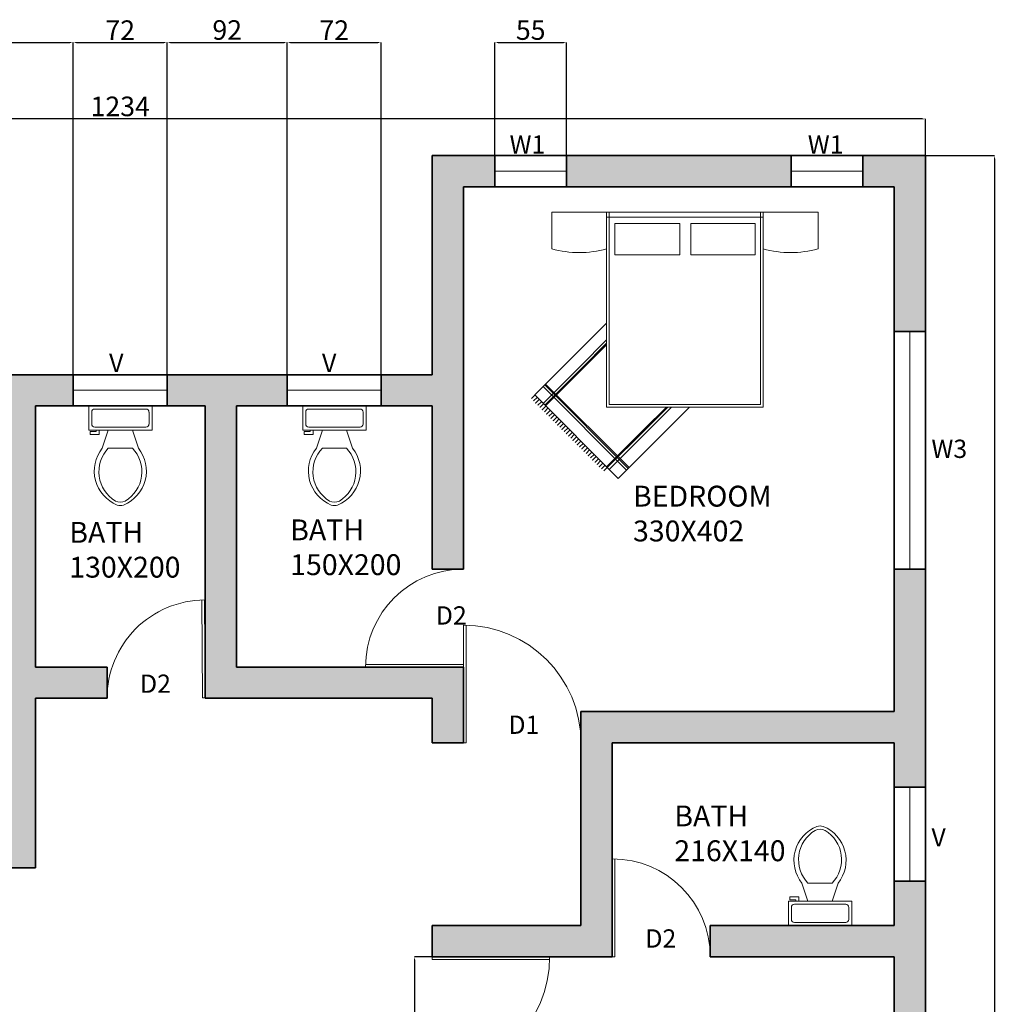
# Model space of a CAD drawing. Units: centimetres. Extents: x 2449 to 7478, y 778 to 2486.
# Tile 9 of 9: x 6695 to 7444, y 1732 to 2486. Entities that reach past the tile are written whole.
import ezdxf

# ---------------------------------------------------------------- set-up
doc = ezdxf.new("R2010")
doc.units = ezdxf.units.CM
for name, color, linetype, lineweight in [('A-ANNO-DIMS', 2, 'Continuous', 18), ('A-ANNO-TEXT', 7, 'Continuous', 18), ('A-AREA-IDEN', 7, 'Continuous', 18), ('A-DOOR', 4, 'Continuous', 18), ('A-FLOR-FIXT', 8, 'Continuous', 18), ('A-WALL', 7, 'Continuous', 35), ('A-WALL-PATT', 7, 'Continuous', 13), ('B-FURNITURE', 22, 'Continuous', 18), ('Win', 1, 'Continuous', 18)]:
    doc.layers.add(name, color=color, linetype=linetype, lineweight=lineweight)
doc.styles.get("Standard").update_dxf_attribs({"font": 'arial.ttf'})
doc.dimstyles.new('ISO-25', dxfattribs={"dimtxt": 15, "dimasz": 2.5, "dimexe": 0, "dimexo": 0, "dimgap": 0, "dimtad": 1, "dimtxsty": 'Standard', "dimcen": 2.5, "dimadec": 0, "dimazin": 0, "dimtfac": 1, "dimtmove": 0, "dimatfit": 3, "dimfxl": 1, "dimarcsym": 0})

# ---------------------------------------------------------------- blocks, each defined once
blk = doc.blocks.new('Toilet - top')
for p, q in [((9.5, -6), (9.5, -2)), ((-10, -8.5), (-8, -8.5)), ((-10, -9.5), (-10, -8.5)), ((-7, -9.5), (-10, -9.5)), ((-8, -8.5), (-8, -8)), ((-7, -8), (-7, -9.5)), ((-4, -8), (-6, -14)), ((4, -8), (6, -14)), ((4, -14), (-4, -14))]:
    blk.add_line(p, q)
blk.add_lwpolyline([(10.5, -8), (10.5, 0), (-10.5, 0), (-10.5, -8)], close=True)
for points in [[(-9.5, -2), (-9.5, -6)], [(8.5, -1), (-8.5, -1)], [(-8.5, -7), (8.5, -7)]]:
    blk.add_lwpolyline(points)
for centre, radius, start, end in [((-8.62, -1.88), 0.884, 81.8699, 188.1301), ((8.62, -1.88), 0.884, 351.8699, 98.1301), ((-8.62, -6.12), 0.884, 171.8699, 278.1301), ((8.62, -6.12), 0.884, 261.8699, 8.1301), ((3.52, -21.58), 12.17, 141.4691, 247.9714), ((4.2, -21.82), 11.33, 136.3677, 238.9468), ((-3.52, -21.58), 12.17, 292.0284, 38.5307), ((-4.2, -21.82), 11.33, 301.053, 43.6321), ((0, -27.88), 4, 245.7318, 294.2682), ((0, -29), 4, 254.8605, 285.1395)]:
    blk.add_arc(centre, radius, start, end)
blk = doc.blocks.new('A$C376C2187')
at = {"layer": 'B-FURNITURE'}
for p, q in [((-1.53, 1.82), (-1.53, 2.24)), ((-1.53, 2.24), (-0.9, 2.24)), ((-0.9, 0), (-0.9, 2.24)), ((-0.9, 2.24), (0.9, 2.24)), ((-0.9, 2.24), (-0.9, 1.82)), ((-0.9, 2.182), (0.9, 2.182)), ((-0.87, 0.03), (-0.87, 2.24)), ((0.87, 2.24), (0.87, 0.03)), ((0.9, 2.24), (0.9, 0)), ((0.9, 1.82), (0.9, 2.24)), ((0.9, 2.24), (1.53, 2.24)), ((1.53, 2.24), (1.53, 1.82)), ((-0.807, 2.112), (-0.057, 2.112)), ((-0.807, 1.749), (-0.807, 2.112)), ((-0.057, 2.112), (-0.057, 1.749)), ((0.069, 2.112), (0.807, 2.112)), ((0.069, 2.112), (0.069, 1.749)), ((0.807, 2.112), (0.807, 1.749)), ((-0.807, 1.749), (-0.057, 1.749)), ((0.069, 1.749), (0.807, 1.749)), ((0.9, 0), (-0.9, 0)), ((0.87, 0.03), (-0.87, 0.03))]:
    blk.add_line(p, q, dxfattribs=at)
for centre in [(-1.215, 2.926), (1.215, 2.926)]:
    blk.add_arc(centre, 1.15, 254.0965, 285.9035, dxfattribs=at)
blk = doc.blocks.new('3')
for p, q in [((5936.31, 1821.57), (5936.31, 1746.57)), ((5938.31, 1821.57), (5938.31, 1746.57)), ((5938.31, 1746.57), (5936.31, 1746.57))]:
    blk.add_line(p, q)
blk.add_arc((5936.31, 1746.57), 75, 0, 90)
blk = doc.blocks.new('2')
for p, q in [((5717.35, 1812.71), (5717.35, 1722.71)), ((5719.35, 1812.71), (5719.35, 1722.71)), ((5719.35, 1722.71), (5717.35, 1722.71))]:
    blk.add_line(p, q)
blk.add_arc((5717.35, 1722.71), 90, 0, 90)
blk = doc.blocks.new('*D63')
at = {"layer": 'A-ANNO-DIMS', "color": 0, "lineweight": -2, "transparency": 16777216}
for p, q in [((6155.01, 2214.34), (6155.01, 2410.3)), ((7386.51, 2410.3), (6157.51, 2410.3)), ((7389.01, 2382.34), (7389.01, 2410.3))]:
    blk.add_line(p, q, dxfattribs=at)
at = {"layer": 'A-ANNO-DIMS', "color": 0, "transparency": 16777216}
for points in [[(6157.51, 2410.71), (6157.51, 2409.88), (6155.01, 2410.3)], [(7386.51, 2410.71), (7386.51, 2409.88), (7389.01, 2410.3)]]:
    blk.add_solid(points, dxfattribs=at)
at = {"layer": 'Defpoints', "color": 0, "transparency": 16777216}
for p in [(6155.01, 2410.3), (7389.01, 2382.34), (6155.01, 2214.34)]:
    blk.add_point(p, dxfattribs=at)
at = {"layer": 'A-ANNO-DIMS', "color": 0, "transparency": 16777216, "insert": (6772.01, 2417.96), "char_height": 15, "attachment_point": 5}
blk.add_mtext('1234', dxfattribs=at)
blk = doc.blocks.new('*D64')
at = {"layer": 'A-ANNO-DIMS', "color": 0, "lineweight": -2, "transparency": 16777216}
for p, q in [((7389.01, 2382.34), (7441.8, 2382.34)), ((7441.8, 2379.84), (7441.8, 1022.84)), ((7389.01, 1020.34), (7441.8, 1020.34))]:
    blk.add_line(p, q, dxfattribs=at)
at = {"layer": 'A-ANNO-DIMS', "color": 0, "transparency": 16777216}
for points in [[(7441.38, 2379.84), (7442.21, 2379.84), (7441.8, 2382.34)], [(7441.38, 1022.84), (7442.21, 1022.84), (7441.8, 1020.34)]]:
    blk.add_solid(points, dxfattribs=at)
at = {"layer": 'Defpoints', "color": 0, "transparency": 16777216}
for p in [(7389.01, 2382.34), (7389.01, 1020.34), (7441.8, 1020.34)]:
    blk.add_point(p, dxfattribs=at)
at = {"layer": 'A-ANNO-DIMS', "color": 0, "transparency": 16777216, "insert": (7434.13, 1701.34), "char_height": 15, "attachment_point": 5, "rotation": 90}
blk.add_mtext('1362', dxfattribs=at)
blk = doc.blocks.new('RUG-FRINGED-A')
for p, q in [((57.64, 119.07), (31.14, 92.56)), ((37.52, 86.17), (57.64, 106.29)), ((38.88, 84.82), (57.64, 103.58)), ((39.46, 84.24), (57.64, 102.42)), ((2.52, 63.95), (31.14, 92.56)), ((37.52, 86.17), (8.91, 57.56)), ((38.88, 84.82), (10.26, 56.2)), ((39.46, 84.24), (10.84, 55.62)), ((72.85, 6.39), (8.91, 70.34)), ((74.21, 7.74), (10.26, 71.69)), ((74.79, 8.33), (10.84, 72.27)), ((2.62, 63.84), (0, 61.22)), ((4.3, 62.16), (1.68, 59.54)), ((66.47, 0), (2.52, 63.95)), ((5.98, 60.48), (3.36, 57.86)), ((7.66, 58.8), (5.04, 56.18)), ((9.34, 57.12), (6.72, 54.5)), ((11.02, 55.44), (8.4, 52.82)), ((12.7, 53.76), (10.08, 51.14)), ((103.41, 54.71), (86.2, 37.5)), ((104.58, 54.71), (86.78, 36.92)), ((107.29, 54.71), (88.14, 35.56)), ((95.08, 28.62), (121.18, 54.71)), ((14.38, 52.08), (11.76, 49.46)), ((16.06, 50.4), (13.44, 47.78)), ((17.74, 48.72), (15.12, 46.1)), ((19.42, 47.04), (16.8, 44.42)), ((21.1, 45.36), (18.48, 42.74)), ((22.78, 43.68), (20.16, 41.06)), ((24.46, 42), (21.84, 39.38)), ((26.14, 40.32), (23.52, 37.7)), ((27.82, 38.64), (25.2, 36.02)), ((29.5, 36.96), (26.88, 34.34)), ((31.18, 35.28), (28.56, 32.66)), ((32.86, 33.6), (30.24, 30.98)), ((34.54, 31.92), (31.92, 29.3)), ((36.22, 30.24), (33.6, 27.62)), ((57.58, 8.88), (86.2, 37.5)), ((58.16, 8.3), (86.78, 36.92)), ((59.52, 6.95), (88.14, 35.56)), ((37.9, 28.56), (35.28, 25.94)), ((39.58, 26.88), (36.96, 24.26)), ((41.26, 25.2), (38.64, 22.58)), ((42.94, 23.52), (40.32, 20.9)), ((95.08, 28.62), (66.47, 0)), ((44.62, 21.84), (42, 19.22)), ((46.3, 20.16), (43.68, 17.54)), ((47.98, 18.48), (45.36, 15.86)), ((49.66, 16.8), (47.04, 14.18)), ((51.34, 15.12), (48.72, 12.5)), ((53.02, 13.44), (50.4, 10.82)), ((54.7, 11.76), (52.08, 9.14)), ((56.38, 10.08), (53.76, 7.46)), ((58.07, 8.4), (55.44, 5.78))]:
    blk.add_line(p, q)
for centre in [(1.62, 59.48), (3.3, 57.8), (4.98, 56.12), (6.66, 54.44), (8.34, 52.76), (10.02, 51.08), (11.7, 49.4), (13.38, 47.72), (15.06, 46.04), (16.74, 44.36), (18.42, 42.68), (20.1, 41), (21.78, 39.32), (23.46, 37.64), (25.14, 35.96), (26.82, 34.28), (28.5, 32.6), (30.18, 30.92), (31.86, 29.24), (33.54, 27.56), (35.22, 25.88), (36.9, 24.2), (38.58, 22.52), (40.26, 20.84), (41.94, 19.16), (43.62, 17.48), (45.3, 15.8), (46.98, 14.12), (48.66, 12.44), (50.34, 10.76), (52.02, 9.08)]:
    blk.add_circle(centre, 0.0789)
blk = doc.blocks.new('*D74')
at = {"layer": 'A-ANNO-DIMS', "color": 0, "lineweight": -2, "transparency": 16777216}
for p, q in [((7011.01, 1768.34), (6997.51, 1768.34)), ((6997.51, 1765.84), (6997.51, 1680.84)), ((7011.01, 1678.34), (6997.51, 1678.34)), ((6997.51, 1678.34), (6997.51, 1502.28))]:
    blk.add_line(p, q, dxfattribs=at)
at = {"layer": 'A-ANNO-DIMS', "color": 0, "transparency": 16777216}
for points in [[(6997.09, 1765.84), (6997.92, 1765.84), (6997.51, 1768.34)], [(6997.09, 1680.84), (6997.92, 1680.84), (6997.51, 1678.34)]]:
    blk.add_solid(points, dxfattribs=at)
at = {"layer": 'Defpoints', "color": 0, "transparency": 16777216}
for p in [(7011.01, 1768.34), (6997.51, 1678.34), (7011.01, 1678.34)]:
    blk.add_point(p, dxfattribs=at)
at = {"layer": 'A-ANNO-DIMS', "color": 0, "transparency": 16777216, "insert": (6989.75, 1589.06), "char_height": 15, "attachment_point": 5, "rotation": 90}
blk.add_mtext('DOOR D1 90 TYP.', dxfattribs=at)
blk = doc.blocks.new('*D109')
at = {"layer": 'A-ANNO-DIMS', "color": 0, "lineweight": -2, "transparency": 16777216}
for p, q in [((6609.01, 2214.34), (6609.01, 2468.84)), ((6611.51, 2468.84), (6733.51, 2468.84)), ((6736.01, 2214.34), (6736.01, 2468.84))]:
    blk.add_line(p, q, dxfattribs=at)
at = {"layer": 'A-ANNO-DIMS', "color": 0, "transparency": 16777216}
for points in [[(6611.51, 2469.26), (6611.51, 2468.42), (6609.01, 2468.84)], [(6733.51, 2469.26), (6733.51, 2468.42), (6736.01, 2468.84)]]:
    blk.add_solid(points, dxfattribs=at)
at = {"layer": 'Defpoints', "color": 0, "transparency": 16777216}
for p in [(6736.01, 2468.84), (6609.01, 2214.34), (6736.01, 2214.34)]:
    blk.add_point(p, dxfattribs=at)
at = {"layer": 'A-ANNO-DIMS', "color": 0, "transparency": 16777216, "insert": (6672.51, 2476.37), "char_height": 15, "attachment_point": 5}
blk.add_mtext('127', dxfattribs=at)
blk = doc.blocks.new('*D110')
at = {"layer": 'A-ANNO-DIMS', "color": 0, "lineweight": -2, "transparency": 16777216}
for p, q in [((6736.01, 2214.34), (6736.01, 2468.84)), ((6738.51, 2468.84), (6805.51, 2468.84)), ((6808.01, 2214.34), (6808.01, 2468.84))]:
    blk.add_line(p, q, dxfattribs=at)
at = {"layer": 'A-ANNO-DIMS', "color": 0, "transparency": 16777216}
for points in [[(6738.51, 2469.26), (6738.51, 2468.42), (6736.01, 2468.84)], [(6805.51, 2469.26), (6805.51, 2468.42), (6808.01, 2468.84)]]:
    blk.add_solid(points, dxfattribs=at)
at = {"layer": 'Defpoints', "color": 0, "transparency": 16777216}
for p in [(6808.01, 2468.84), (6736.01, 2214.34), (6808.01, 2214.34)]:
    blk.add_point(p, dxfattribs=at)
at = {"layer": 'A-ANNO-DIMS', "color": 0, "transparency": 16777216, "insert": (6772.01, 2476.37), "char_height": 15, "attachment_point": 5}
blk.add_mtext('72', dxfattribs=at)
blk = doc.blocks.new('*D111')
at = {"layer": 'A-ANNO-DIMS', "color": 0, "lineweight": -2, "transparency": 16777216}
for p, q in [((6808.01, 2214.34), (6808.01, 2468.84)), ((6810.51, 2468.84), (6897.51, 2468.84)), ((6900.01, 2214.34), (6900.01, 2468.84))]:
    blk.add_line(p, q, dxfattribs=at)
at = {"layer": 'A-ANNO-DIMS', "color": 0, "transparency": 16777216}
for points in [[(6810.51, 2469.26), (6810.51, 2468.42), (6808.01, 2468.84)], [(6897.51, 2469.26), (6897.51, 2468.42), (6900.01, 2468.84)]]:
    blk.add_solid(points, dxfattribs=at)
at = {"layer": 'Defpoints', "color": 0, "transparency": 16777216}
for p in [(6900.01, 2468.84), (6808.01, 2214.34), (6900.01, 2214.34)]:
    blk.add_point(p, dxfattribs=at)
at = {"layer": 'A-ANNO-DIMS', "color": 0, "transparency": 16777216, "insert": (6854.01, 2476.5), "char_height": 15, "attachment_point": 5}
blk.add_mtext('92', dxfattribs=at)
blk = doc.blocks.new('*D112')
at = {"layer": 'A-ANNO-DIMS', "color": 0, "lineweight": -2, "transparency": 16777216}
for p, q in [((6900.01, 2214.34), (6900.01, 2468.84)), ((6902.51, 2468.84), (6969.51, 2468.84)), ((6972.01, 2214.34), (6972.01, 2468.84))]:
    blk.add_line(p, q, dxfattribs=at)
at = {"layer": 'A-ANNO-DIMS', "color": 0, "transparency": 16777216}
for points in [[(6902.51, 2469.26), (6902.51, 2468.42), (6900.01, 2468.84)], [(6969.51, 2469.26), (6969.51, 2468.42), (6972.01, 2468.84)]]:
    blk.add_solid(points, dxfattribs=at)
at = {"layer": 'Defpoints', "color": 0, "transparency": 16777216}
for p in [(6972.01, 2468.84), (6900.01, 2214.34), (6972.01, 2214.34)]:
    blk.add_point(p, dxfattribs=at)
at = {"layer": 'A-ANNO-DIMS', "color": 0, "transparency": 16777216, "insert": (6936.01, 2476.37), "char_height": 15, "attachment_point": 5}
blk.add_mtext('72', dxfattribs=at)
blk = doc.blocks.new('*D113')
at = {"layer": 'A-ANNO-DIMS', "color": 0, "lineweight": -2, "transparency": 16777216}
for p, q in [((7059.01, 2382.34), (7059.01, 2468.84)), ((7061.51, 2468.84), (7111.51, 2468.84)), ((7114.01, 2382.34), (7114.01, 2468.84))]:
    blk.add_line(p, q, dxfattribs=at)
at = {"layer": 'A-ANNO-DIMS', "color": 0, "transparency": 16777216}
for points in [[(7061.51, 2469.26), (7061.51, 2468.42), (7059.01, 2468.84)], [(7111.51, 2469.26), (7111.51, 2468.42), (7114.01, 2468.84)]]:
    blk.add_solid(points, dxfattribs=at)
at = {"layer": 'Defpoints', "color": 0, "transparency": 16777216}
for p in [(7114.01, 2468.84), (7059.01, 2382.34), (7114.01, 2382.34)]:
    blk.add_point(p, dxfattribs=at)
at = {"layer": 'A-ANNO-DIMS', "color": 0, "transparency": 16777216, "insert": (7086.51, 2476.47), "char_height": 15, "attachment_point": 5}
blk.add_mtext('55', dxfattribs=at)

msp = doc.modelspace()

# ---------------------------------------------------------------- hatches: boundary and pattern name
at = {"layer": 'A-WALL-PATT'}
h = msp.add_hatch(color=256, dxfattribs=at)
h.dxf.hatch_style = 1
h.paths.add_polyline_path([(6637.006, 1092.34), (6563.006, 1092.34), (6563.006, 1068.34), (6661.006, 1068.34), (6661.006, 1476.34), (6637.006, 1476.34)])
h.paths.add_polyline_path([(6283.006, 1167.34), (6307.006, 1167.34), (6307.006, 1377.34), (6283.006, 1377.34)])
h.paths.add_polyline_path([(6381.006, 1068.34), (6381.006, 1092.34), (6307.006, 1092.34), (6307.006, 1112.34), (6283.006, 1112.34), (6283.006, 1068.34)])
h.paths.add_polyline_path([(6307.006, 1551.34), (6283.006, 1551.34), (6283.006, 1432.34), (6307.006, 1432.34), (6307.006, 1452.34), (6547.006, 1452.34), (6547.006, 1476.34), (6307.006, 1476.34)])
h.paths.add_polyline_path([(7011.006, 1654.34), (7011.006, 1266.34), (6982.006, 1266.34), (6982.006, 1242.34), (7035.006, 1242.34), (7035.006, 1404.34), (7059.006, 1404.34), (7059.006, 1428.34), (7035.006, 1428.34), (7035.006, 1678.34), (6837.006, 1678.34), (6837.006, 1654.34)])
h.paths.add_polyline_path([(6800.006, 1266.34), (6771.006, 1266.34), (6771.006, 1242.34), (6800.006, 1242.34)])
h.paths.add_polyline_path([(7389.006, 1506.339), (7365.006, 1506.339), (7365.006, 1428.34), (7341.006, 1428.34), (7341.006, 1404.34), (7389.006, 1404.34)])
h.paths.add_polyline_path([(7286.006, 1404.34), (7286.006, 1428.34), (7114.006, 1428.34), (7114.006, 1404.34)])
h.paths.add_polyline_path([(7365.006, 1688.339), (7389.006, 1688.339), (7389.006, 1826.34), (7365.006, 1826.34), (7365.006, 1792.34), (7224.006, 1792.34), (7224.006, 1768.34), (7365.006, 1768.34)])
h.paths.add_polyline_path([(7365.006, 1956.34), (7125.006, 1956.34), (7125.006, 1792.34), (7011.006, 1792.34), (7011.006, 1768.34), (7149.006, 1768.34), (7149.006, 1932.34), (7365.006, 1932.34), (7365.006, 1898.34), (7389.006, 1898.34), (7389.006, 2065.339), (7365.006, 2065.339)])
h.paths.add_polyline_path([(7365.006, 2358.34), (7365.006, 2247.339), (7389.006, 2247.339), (7389.006, 2382.34), (7341.006, 2382.34), (7341.006, 2358.34)])
h.paths.add_polyline_path([(7114.006, 2382.34), (7114.006, 2358.34), (7286.006, 2358.34), (7286.006, 2382.34)])
h.paths.add_polyline_path([(7035.006, 2358.34), (7059.006, 2358.34), (7059.006, 2382.34), (7011.006, 2382.34), (7011.006, 2214.34), (6972.006, 2214.34), (6972.006, 2190.34), (7011.006, 2190.34), (7011.006, 2065.34), (7035.006, 2065.34)])
h.paths.add_polyline_path([(6808.006, 2214.34), (6808.006, 2190.34), (6837.006, 2190.34), (6837.006, 1966.34), (7011.006, 1966.34), (7011.006, 1932.34), (7035.006, 1932.34), (7035.006, 1990.34), (6861.006, 1990.34), (6861.006, 2190.34), (6900.006, 2190.34), (6900.006, 2214.34)])
h.paths.add_polyline_path([(6707.006, 2190.34), (6736.006, 2190.34), (6736.006, 2214.34), (6609.006, 2214.34), (6609.006, 2190.34), (6683.006, 2190.34), (6683.006, 1836.34), (6707.006, 1836.34), (6707.006, 1966.34), (6762.006, 1966.34), (6762.006, 1990.34), (6707.006, 1990.34)])
h.paths.add_polyline_path([(6315.006, 2214.34), (6315.006, 2190.34), (6329.006, 2190.34), (6329.006, 1935.34), (6353.006, 1935.34), (6353.006, 2190.34), (6427.006, 2190.34), (6427.006, 2214.34)])
h.paths.add_polyline_path([(6155.006, 2152.839), (6179.006, 2152.839), (6179.006, 2190.34), (6193.006, 2190.34), (6193.006, 2214.34), (6155.006, 2214.34)])
h.paths.add_polyline_path([(6155.006, 1935.34), (6179.006, 1935.34), (6179.006, 1970.839), (6155.006, 1970.839)])
h.paths.add_polyline_path([(6283.006, 1836.34), (6283.006, 1791.34), (6307.006, 1791.34), (6307.006, 1836.34), (6593.006, 1836.34), (6593.006, 1860.34), (6155.006, 1860.34), (6155.006, 1836.34)])

# ---------------------------------------------------------------- linework, layer by layer
at = {"layer": 'A-WALL'}
for p, q in [((7011.006, 2382.34), (7389.006, 2382.34)), ((7011.006, 2214.34), (7011.006, 2382.34)), ((7059.006, 2382.34), (7059.006, 2358.34)), ((7114.006, 2382.34), (7114.006, 2358.34)), ((7286.006, 2382.34), (7286.006, 2358.34)), ((7341.006, 2382.34), (7341.006, 2358.34)), ((7389.006, 2382.34), (7389.006, 1020.34)), ((7035.006, 2358.34), (7035.006, 2065.34)), ((7035.006, 2358.34), (7365.006, 2358.34)), ((7365.006, 2358.34), (7365.006, 1956.34)), ((7365.006, 2247.339), (7389.006, 2247.339)), ((6155.006, 2214.34), (7011.006, 2214.34)), ((6736.006, 2190.34), (6736.006, 2214.34)), ((6808.006, 2190.34), (6808.006, 2214.34)), ((6900.006, 2190.34), (6900.006, 2214.34)), ((6972.006, 2190.34), (6972.006, 2214.34)), ((6707.006, 2190.34), (6837.006, 2190.34)), ((6707.006, 2190.34), (6707.006, 1990.34)), ((6837.006, 2190.34), (6837.006, 1966.34)), ((6861.006, 2190.34), (7011.006, 2190.34)), ((6861.006, 2190.34), (6861.006, 1990.34)), ((7011.006, 2190.34), (7011.006, 2065.34)), ((7011.006, 2065.34), (7035.006, 2065.34)), ((7365.006, 2065.339), (7389.006, 2065.339)), ((6707.006, 1990.34), (6762.006, 1990.34)), ((6762.006, 1990.34), (6762.006, 1966.34)), ((6861.006, 1990.34), (7035.006, 1990.34)), ((7035.006, 1990.34), (7035.006, 1932.34)), ((6707.006, 1966.34), (6762.006, 1966.34)), ((6707.006, 1966.34), (6707.006, 1836.34)), ((6837.006, 1966.34), (7011.006, 1966.34)), ((7011.006, 1966.34), (7011.006, 1932.34)), ((7125.006, 1956.34), (7365.006, 1956.34)), ((7125.006, 1956.34), (7125.006, 1792.34)), ((7011.006, 1932.34), (7035.006, 1932.34)), ((7149.006, 1932.34), (7365.006, 1932.34)), ((7149.006, 1932.34), (7149.006, 1768.34)), ((7365.006, 1932.34), (7365.006, 1792.34)), ((7365.006, 1898.34), (7389.006, 1898.34)), ((6683.006, 1836.34), (6707.006, 1836.34)), ((7365.006, 1826.34), (7389.006, 1826.34)), ((7011.006, 1792.34), (7011.006, 1768.34)), ((7011.006, 1792.34), (7125.006, 1792.34)), ((7224.006, 1792.34), (7365.006, 1792.34)), ((7224.006, 1792.34), (7224.006, 1768.34)), ((7011.006, 1768.34), (7149.006, 1768.34)), ((7224.006, 1768.34), (7365.006, 1768.34)), ((7365.006, 1768.34), (7365.006, 1428.34))]:
    msp.add_line(p, q, dxfattribs=at)
at = {"layer": 'Win'}
for p, q in [((7059.006, 2370.34), (7114.006, 2370.34)), ((7286.006, 2370.34), (7341.006, 2370.34)), ((7377.006, 2247.339), (7377.006, 2065.339)), ((6808.006, 2202.34), (6736.006, 2202.34)), ((6972.006, 2202.34), (6900.006, 2202.34)), ((7377.006, 1898.34), (7377.006, 1826.34))]:
    msp.add_line(p, q, dxfattribs=at)

# ---------------------------------------------------------------- block references
at = {"layer": 'A-DOOR'}
for name, p, rotation in [('3', (8781.573, -3945.97), 90), ('2', (5288.291, 7485.689), 270)]:
    msp.add_blockref(name, p, dxfattribs=dict(at, rotation=rotation))
at = {"layer": 'A-DOOR', "xscale": -1, "rotation": 0.2708478329988573}
msp.add_blockref('3', (12781.505, 248.208), dxfattribs=at)
at = {"layer": 'A-DOOR'}
for name, p in [('2', (1317.657, 209.625)), ('3', (1212.696, 21.772))]:
    msp.add_blockref(name, p, dxfattribs=at)
at = {"layer": 'A-FLOR-FIXT', "xscale": 2.309305753348624, "yscale": 2.309305753348624, "zscale": 2.309305753348624}
for p in [(6772.133, 2190.34), (6936.133, 2190.34)]:
    msp.add_blockref('Toilet - top', p, dxfattribs=at)
at = {"layer": 'A-FLOR-FIXT', "xscale": -2.309305753348624, "yscale": 2.309305753348624, "zscale": 2.309305753348624, "rotation": 180}
msp.add_blockref('Toilet - top', (7308.176, 1792.34), dxfattribs=at)
at = {"layer": 'B-FURNITURE', "xscale": 66.63496932822166, "yscale": 66.63496932822166, "zscale": 66.63496932822166}
msp.add_blockref('A$C376C2187', (7204.656, 2189.525), dxfattribs=at)
at = {"layer": 'B-FURNITURE'}
msp.add_blockref('RUG-FRINGED-A', (7087.047, 2134.812), dxfattribs=at)

# ---------------------------------------------------------------- texts
at = {"layer": 'A-ANNO-TEXT', "char_height": 14, "attachment_point": 1}
for s, insert in [('{\\fTimes New Roman|b0|i0|c0|p18;\\PW1}', (7070.343, 2421.005)), ('{\\fTimes New Roman|b0|i0|c0|p18;\\PW1}', (7298.784, 2421.005)), ('{\\fTimes New Roman|b0|i0|c0|p18;\\P   V}', (6750.694, 2253.652)), ('{\\fTimes New Roman|b0|i0|c0|p18;\\P   V}', (6913.785, 2253.652)), ('{\\fTimes New Roman|b0|i0|c0|p18;\\PW3}', (7393.512, 2187.869)), ('{\\fTimes New Roman|b0|i0|c0|p18;\\PD2}', (7013.779, 2060.184)), ('{\\fTimes New Roman|b0|i0|c0|p18;\\PD2}', (6787.155, 2007.896)), ('{\\fTimes New Roman|b0|i0|c0|p18;\\PD1}', (7069.437, 1976.446)), ('{\\fTimes New Roman|b0|i0|c0|p18;\\PV}', (7393.512, 1890.156)), ('{\\fTimes New Roman|b0|i0|c0|p18;\\PD2}', (7174.295, 1812.646))]:
    msp.add_mtext_dynamic_manual_height_columns(s, width=211.90348, gutter_width=12.5, heights=[0], dxfattribs=dict(at, insert=insert))
at = {"layer": 'A-AREA-IDEN', "char_height": 16, "attachment_point": 1}
for s, insert in [('{\\fTimes New Roman|b0|i0|c0|p18;\\PBEDROOM           330X402}', (7164.901, 2155.913)), ('{\\fTimes New Roman|b0|i0|c0|p18;\\PBATH\\P130X200}', (6733.01, 2128.174)), ('{\\fTimes New Roman|b0|i0|c0|p18;\\PBATH\\P150X200}', (6902.245, 2130.078)), ('{\\fTimes New Roman|b0|i0|c0|p18;\\PBATH\\P216X140}', (7196.526, 1910.877))]:
    msp.add_mtext_dynamic_manual_height_columns(s, width=211.90348, gutter_width=12.5, heights=[0], dxfattribs=dict(at, insert=insert))

# ---------------------------------------------------------------- dimensions: what is measured, and where the dimension line sits
at = {"layer": 'A-ANNO-DIMS'}
for base, p1, p2, override, picture, middle in [((6736.006, 2468.84), (6609.006, 2214.34), (6736.006, 2214.34), {"dimdec": 0, "dimlfac": 1, "dimrnd": 0, "dimzin": 0, "dimdsep": 46, "dimlunit": 2}, '*D109', (6672.506, 2476.37)), ((6808.006, 2468.84), (6736.006, 2214.34), (6808.006, 2214.34), {"dimdec": 0, "dimlfac": 1, "dimrnd": 0, "dimzin": 0, "dimdsep": 46, "dimlunit": 2}, '*D110', (6772.006, 2476.37)), ((6900.006, 2468.84), (6808.006, 2214.34), (6900.006, 2214.34), {"dimdec": 0, "dimlfac": 1, "dimrnd": 0, "dimzin": 0, "dimdsep": 46, "dimlunit": 2}, '*D111', (6854.006, 2476.498)), ((6972.006, 2468.84), (6900.006, 2214.34), (6972.006, 2214.34), {"dimdec": 0, "dimlfac": 1, "dimrnd": 0, "dimzin": 0, "dimdsep": 46, "dimlunit": 2}, '*D112', (6936.006, 2476.37)), ((7114.006, 2468.84), (7059.006, 2382.34), (7114.006, 2382.34), {"dimdec": 0, "dimlfac": 1, "dimrnd": 0, "dimzin": 0, "dimdsep": 46, "dimlunit": 2}, '*D113', (7086.506, 2476.468)), ((6155.006, 2410.295), (7389.006, 2382.34), (6155.006, 2214.34), {"dimclrd": 0, "dimclre": 0, "dimclrt": 0}, '*D63', (6772.006, 2417.959))]:
    dim = msp.add_linear_dim(base=base, p1=p1, p2=p2, dimstyle='ISO-25', override=override, dxfattribs=at)
    dim.commit()
    dim.dimension.update_dxf_attribs({"geometry": picture, "text_midpoint": middle})
dim = msp.add_linear_dim(base=(7441.795, 1020.34), p1=(7389.006, 2382.34), p2=(7389.006, 1020.34), angle=90, dimstyle='ISO-25', override={"dimclrd": 0, "dimclre": 0, "dimclrt": 0}, dxfattribs=at)
dim.commit()
dim.dimension.update_dxf_attribs({"geometry": '*D64', "text_midpoint": (7434.132, 1701.34)})
dim = msp.add_linear_dim(base=(6997.506, 1678.34), p1=(7011.006, 1768.34), p2=(7011.006, 1678.34), angle=270, text='DOOR D1 <> TYP.', dimstyle='ISO-25', override={"dimdec": 0, "dimlfac": 1, "dimrnd": 0, "dimzin": 0, "dimdsep": 46, "dimlunit": 2}, dxfattribs=at)
dim.commit()
dim.dimension.update_dxf_attribs({"geometry": '*D74', "text_midpoint": (6989.745, 1589.058)})

doc.saveas('drawing.dxf')
